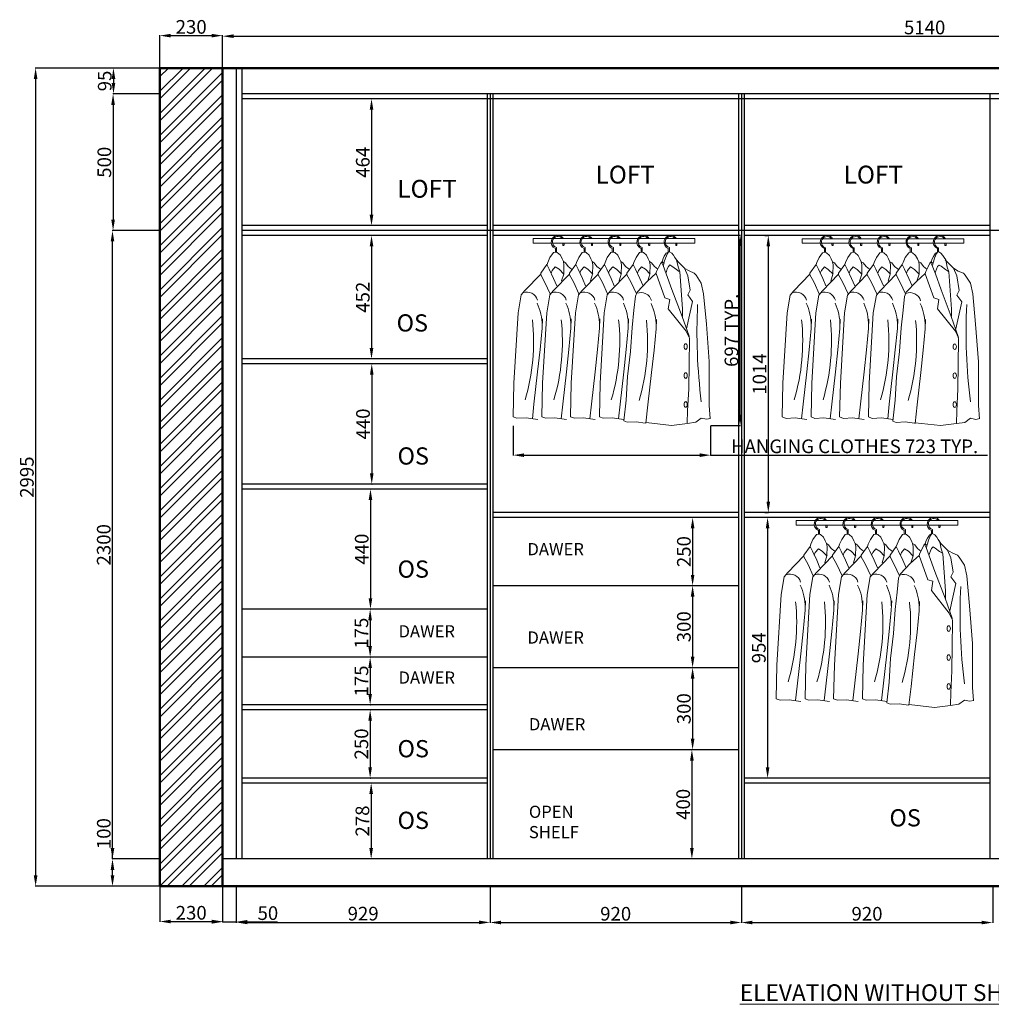
# Model space of a CAD drawing. Units: millimetres. Extents: x -513 to 5600, y -432 to 3172.
# Tile 1 of 2: x -513 to 3044, y -432 to 3172. Entities that reach past the tile are written whole.
import ezdxf

# ---------------------------------------------------------------- set-up
doc = ezdxf.new("R2010")
doc.units = ezdxf.units.MM
for name, color, linetype, lineweight in [('A-ANNO-DIMS', 2, 'Continuous', 18), ('A-ANNO-TEXT', 7, 'Continuous', 18), ('A-FURN', 3, 'Continuous', 25), ('A-FURN-ACCS', 9, 'Continuous', 18), ('A-WALL', 7, 'Continuous', 50), ('A-WALL-PATT', 8, 'Continuous', 13)]:
    doc.layers.add(name, color=color, linetype=linetype, lineweight=lineweight)
doc.styles.get("Standard").update_dxf_attribs({"font": 'arial.ttf'})
doc.dimstyles.new('ISO-25', dxfattribs={"dimtxt": 50, "dimasz": 40, "dimexe": 1.25, "dimexo": 0.625, "dimgap": 0, "dimtad": 1, "dimtxsty": 'Standard', "dimcen": 2.5, "dimclrt": 6, "dimadec": 0, "dimazin": 0, "dimtfac": 1, "dimtmove": 0, "dimatfit": 3, "dimfxl": 1, "dimarcsym": 0})

# ---------------------------------------------------------------- blocks, each defined once
blk = doc.blocks.new('A$C17AF523A')
for p, q in [((221.1, 1060), (113.2, 1060)), ((113.2, 1060), (113.2, 1034.3)), ((216, 1034.3), (113.2, 1034.3)), ((222.5, 1034.3), (378.4, 1034.3)), ((229, 1060), (383.5, 1060)), ((246.1, 1008.9), (246.1, 981.5)), ((285.8, 1060), (336.5, 1060)), ((384.9, 1034.3), (538.6, 1034.3)), ((391.4, 1060), (543.8, 1060)), ((408.5, 1008.9), (408.5, 981.5)), ((545.2, 1034.3), (702.4, 1034.3)), ((551.6, 1060), (707.5, 1060)), ((568.8, 1008.9), (568.8, 981.5)), ((708.9, 1034.3), (856.3, 1034.3)), ((715.4, 1060), (861.4, 1060)), ((732.5, 1008.9), (732.5, 982.4)), ((862.8, 1034.3), (1030.4, 1034.3)), ((869.3, 1060), (1030.4, 1060)), ((886.4, 1008.9), (886.4, 985.5)), ((1030.4, 1060), (1030.4, 1034.3)), ((208.5, 953.2), (196.2, 925.3)), ((228.2, 980.3), (208.5, 953.2)), ((240.6, 982.7), (228.2, 980.3)), ((239.7, 981.5), (239.7, 1004.2)), ((250.4, 980.3), (240.6, 982.7)), ((267.7, 965.5), (250.4, 980.3)), ((277.5, 945), (267.7, 965.5)), ((371.7, 953.2), (359.4, 925.3)), ((391.4, 980.3), (371.7, 953.2)), ((403.7, 982.7), (391.4, 980.3)), ((402.1, 981.5), (402.1, 1004.2)), ((413.6, 980.3), (403.7, 982.7)), ((430.8, 965.5), (413.6, 980.3)), ((440.7, 945), (430.8, 965.5)), ((534.1, 953.2), (521.8, 925.3)), ((553.8, 980.3), (534.1, 953.2)), ((566.1, 982.7), (553.8, 980.3)), ((562.3, 981.5), (562.3, 1004.2)), ((576, 980.3), (566.1, 982.7)), ((593.2, 965.5), (576, 980.3)), ((603.1, 945), (593.2, 965.5)), ((697.3, 953.2), (685, 925.3)), ((717, 980.3), (697.3, 953.2)), ((729.3, 982.7), (717, 980.3)), ((726.1, 981.9), (726.1, 1004.2)), ((739.2, 980.3), (729.3, 982.7)), ((756.4, 965.5), (739.2, 980.3)), ((766.3, 945), (756.4, 965.5)), ((857, 959.7), (850.7, 946.2)), ((868.4, 977.4), (857, 959.7)), ((864.2, 949.2), (857, 928.1)), ((874.7, 975.3), (864.2, 949.2)), ((881.5, 985.8), (868.4, 977.4)), ((881.5, 985.8), (874.7, 975.3)), ((880, 984.9), (880, 1004.2)), ((887.4, 985), (881.5, 985.8)), ((899.2, 978.2), (887.4, 985)), ((910.2, 965.2), (899.2, 978.2)), ((917.7, 953.4), (910.2, 965.2)), ((927, 940.3), (917.7, 953.4)), ((192, 913.2), (156.7, 863.9)), ((204.9, 887.4), (192, 913.2)), ((196.2, 925.3), (192.1, 913)), ((238.9, 899.8), (221.7, 879.3)), ((261.1, 885.9), (238.9, 899.8)), ((284.9, 929.7), (277.5, 945)), ((296.7, 922.6), (284.9, 929.7)), ((284.9, 929.7), (288.4, 912.1)), ((288.4, 912.1), (287.3, 859.2)), ((312, 901.5), (296.7, 922.6)), ((331.5, 886.8), (312, 901.5)), ((355.1, 913.2), (319.8, 863.9)), ((368.1, 887.4), (355.1, 913.2)), ((359.4, 925.3), (355.3, 913)), ((402.1, 899.8), (384.8, 879.3)), ((424.3, 885.9), (402.1, 899.8)), ((448.1, 929.7), (440.7, 945)), ((459.8, 922.6), (448.1, 929.7)), ((448.1, 929.7), (451.6, 912.1)), ((451.6, 912.1), (450.4, 859.2)), ((475.1, 901.5), (459.8, 922.6)), ((494.7, 886.8), (475.1, 901.5)), ((517.5, 913.2), (482.2, 863.9)), ((530.5, 887.4), (517.5, 913.2)), ((521.8, 925.3), (517.7, 913)), ((564.5, 899.8), (547.2, 879.3)), ((586.7, 885.9), (564.5, 899.8)), ((610.5, 929.7), (603.1, 945)), ((622.3, 922.6), (610.5, 929.7)), ((610.5, 929.7), (614, 912.1)), ((614, 912.1), (612.8, 859.2)), ((637.5, 901.5), (622.3, 922.6)), ((657.1, 886.8), (637.5, 901.5)), ((680.7, 913.2), (645.4, 863.9)), ((693.6, 887.4), (680.7, 913.2)), ((685, 925.3), (680.8, 913)), ((727.7, 899.8), (710.4, 879.3)), ((749.8, 885.9), (727.7, 899.8)), ((773.7, 929.7), (766.3, 945)), ((785.4, 922.6), (773.7, 929.7)), ((773.7, 929.7), (777.2, 912.1)), ((777.2, 912.1), (776, 859.2)), ((800.7, 901.5), (785.4, 922.6)), ((820.3, 886.8), (800.7, 901.5)), ((813.7, 874.2), (824.9, 895.9)), ((824.9, 895.9), (837.6, 920.5)), ((837.6, 920.5), (842.9, 928.7)), ((841.4, 926.4), (851.1, 907.8)), ((842.9, 928.7), (854, 920.5)), ((850.7, 946.2), (844.4, 926.4)), ((851.1, 907.8), (868.2, 860.1)), ((852.8, 910), (852.4, 907.5)), ((857, 928.1), (852.8, 910)), ((854, 920.5), (855.5, 919.7)), ((881.1, 902.4), (873.9, 888.1)), ((889.5, 910.4), (881.1, 902.4)), ((900.5, 903.7), (889.5, 910.4)), ((925.8, 885.1), (900.5, 903.7)), ((938.9, 924.4), (924.5, 940.7)), ((927, 940.3), (935.1, 899.5)), ((935.1, 899.5), (944.7, 871.7)), ((971.6, 892.8), (938.9, 924.4)), ((156.7, 859.2), (66.1, 765.1)), ((180.6, 811.5), (154.8, 858.5)), ((156.7, 863.9), (156.7, 859.2)), ((229.6, 834.5), (204.9, 887.4)), ((221.7, 879.3), (215.7, 864.3)), ((319.8, 859.2), (229.2, 765.1)), ((288.2, 858.8), (261.1, 885.9)), ((287.3, 859.2), (275, 820)), ((343.8, 811.5), (317.9, 858.5)), ((319.8, 863.9), (319.8, 859.2)), ((392.8, 834.5), (368.1, 887.4)), ((384.8, 879.3), (378.8, 864.3)), ((482.2, 859.2), (391.6, 765.1)), ((451.4, 858.8), (424.3, 885.9)), ((450.4, 859.2), (438.2, 820)), ((506.2, 811.5), (480.3, 858.5)), ((482.2, 863.9), (482.2, 859.2)), ((555.2, 834.5), (530.5, 887.4)), ((547.2, 879.3), (541.2, 864.3)), ((645.4, 859.2), (554.8, 765.1)), ((613.8, 858.8), (586.7, 885.9)), ((612.8, 859.2), (600.6, 820)), ((669.4, 811.5), (643.5, 858.5)), ((645.4, 863.9), (645.4, 859.2)), ((718.4, 834.5), (693.6, 887.4)), ((710.4, 879.3), (704.4, 864.3)), ((776.9, 858.8), (749.8, 885.9)), ((761.8, 818.2), (810, 862)), ((776, 859.2), (763.8, 820)), ((810, 862), (813.7, 874.2)), ((859.8, 724), (811, 861.6)), ((869.3, 872.5), (867.6, 867)), ((868.2, 860.1), (900.3, 770.6)), ((873.9, 888.1), (869.3, 872.5)), ((942.2, 874.2), (925.8, 885.1)), ((944.7, 871.7), (960, 660.8)), ((970.6, 892.8), (997.5, 876.5)), ((989.8, 849.6), (971.6, 892.8)), ((1004.2, 767.2), (989.8, 849.6)), ((997.5, 876.5), (1027.2, 864)), ((1027.2, 864), (1037.8, 852.5)), ((1037.8, 852.5), (1067.2, 807.9)), ((210.3, 746.9), (180.6, 811.5)), ((247.8, 792.1), (229.6, 834.5)), ((373.4, 746.9), (343.8, 811.5)), ((411, 792.1), (392.8, 834.5)), ((535.8, 746.9), (506.2, 811.5)), ((573.4, 792.1), (555.2, 834.5)), ((699, 746.9), (669.4, 811.5)), ((702.6, 756.9), (761.8, 818.2)), ((736.6, 792.1), (718.4, 834.5)), ((1067.2, 807.9), (1080, 746.6)), ((44.9, 740.4), (27.8, 639.9)), ((66.1, 765.1), (44.9, 740.4)), ((208, 740.4), (190.9, 639.9)), ((229.2, 765.1), (208, 740.4)), ((370.5, 740.4), (353.3, 639.9)), ((391.6, 765.1), (370.5, 740.4)), ((533.6, 740.4), (516.5, 639.9)), ((554.8, 765.1), (533.6, 740.4)), ((685.1, 654), (693.9, 732.8)), ((693.9, 732.8), (702.6, 756.9)), ((900.3, 770.6), (958.5, 619.2)), ((990.7, 740.3), (1004.2, 767.2)), ((1017.6, 702.9), (990.7, 740.3)), ((1080, 746.6), (1096.5, 575.6)), ((888.4, 715.5), (859.8, 724)), ((879.9, 662.5), (888.4, 715.5)), ((984, 548.6), (1017.6, 702.9)), ((27.8, 639.9), (4.2, 240.5)), ((190.9, 639.9), (167.4, 240.5)), ((353.3, 639.9), (329.8, 240.5)), ((516.5, 639.9), (493, 240.5)), ((674.2, 555.5), (685.1, 654)), ((981.6, 535.4), (879.9, 662.5)), ((958.5, 619.2), (997.3, 506.4)), ((960, 660.8), (960, 618.6)), ((163.9, 551.6), (166.2, 604.3)), ((327.1, 551.6), (329.4, 604.3)), ((489.5, 551.6), (491.8, 604.3)), ((652.7, 551.6), (655, 604.3)), ((810.2, 548.7), (812.5, 601.4)), ((1096.5, 575.6), (1112.5, 362.3)), ((152.5, 430.3), (163.9, 551.6)), ((315.7, 430.3), (327.1, 551.6)), ((478.1, 430.3), (489.5, 551.6)), ((641.2, 430.3), (652.7, 551.6)), ((665.4, 419.8), (674.2, 555.5)), ((798.8, 427.4), (810.2, 548.7)), ((998.6, 498.4), (981.6, 535.4)), ((997.3, 506.4), (1000, 487.4)), ((1000, 487.4), (996.4, 208.2)), ((138.7, 304.3), (152.5, 430.3)), ((301.9, 304.3), (315.7, 430.3)), ((464.3, 304.3), (478.1, 430.3)), ((627.5, 304.3), (641.2, 430.3)), ((647.9, 277.5), (665.4, 419.8)), ((785, 301.4), (798.8, 427.4)), ((1112.5, 362.3), (1112.5, 113.9)), ((118.1, 121.1), (138.7, 304.3)), ((281.3, 121.1), (301.9, 304.3)), ((443.7, 121.1), (464.3, 304.3)), ((606.9, 121.1), (627.5, 304.3)), ((764.4, 118.2), (785, 301.4)), ((4.2, 240.5), (0, 49.5)), ((167.4, 240.5), (163.2, 49.5)), ((329.8, 240.5), (325.6, 49.5)), ((493, 240.5), (488.8, 49.5)), ((641.3, 143.9), (647.9, 277.5)), ((996.4, 208.2), (989.7, 82.6)), ((109.2, 38.9), (118.1, 121.1)), ((272.3, 38.9), (281.3, 121.1)), ((434.7, 38.9), (443.7, 121.1)), ((597.9, 38.9), (606.9, 121.1)), ((627.3, 25.8), (641.3, 143.9)), ((752.9, 12.8), (764.4, 118.2)), ((1112.5, 113.9), (1118.2, 39.6)), ((989.7, 82.6), (987.5, 14.7)), ((21.7, 41.4), (0, 49.5)), ((73.3, 43.8), (21.7, 41.4)), ((139.6, 34.7), (73.3, 43.8)), ((184.8, 41.4), (163.2, 49.5)), ((236.5, 43.8), (184.8, 41.4)), ((302.8, 34.7), (236.5, 43.8)), ((347.2, 41.4), (325.6, 49.5)), ((398.9, 43.8), (347.2, 41.4)), ((465.2, 34.7), (398.9, 43.8)), ((510.4, 41.4), (488.8, 49.5)), ((562.1, 43.8), (510.4, 41.4)), ((628.3, 34.7), (562.1, 43.8)), ((646.1, 18.8), (627.3, 25.8)), ((697.8, 21.1), (646.1, 18.8)), ((749.5, 14.1), (697.8, 21.1)), ((754.2, 16.4), (897.4, 0)), ((897.4, 0), (989, 11.7)), ((989, 11.7), (1036, 18.8)), ((1036, 18.8), (1067.2, 42.2)), ((1067.2, 42.2), (1096.9, 35.3)), ((1096.9, 35.3), (1119.7, 39.9))]:
    blk.add_line(p, q)
for centre, radius, start, end in [((253.5, 1040.3), 37.9, 31.4138, 165.4823), ((253.5, 1040.3), 31.5, 38.898, 165.4823), ((415.9, 1040.3), 37.9, 31.4138, 165.4823), ((415.9, 1040.3), 31.5, 38.898, 165.4823), ((576.1, 1040.3), 37.9, 31.4138, 165.4823), ((576.1, 1040.3), 31.5, 38.898, 165.4823), ((739.9, 1040.3), 37.9, 31.4138, 165.4823), ((739.9, 1040.3), 31.5, 38.898, 165.4823), ((893.8, 1040.3), 37.9, 31.4138, 165.4823), ((893.8, 1040.3), 31.5, 38.898, 165.4823), ((254.3, 1040.1), 38.7, 165.4823, 247.8669), ((254.3, 1040.1), 32.3, 165.4823, 255.3823), ((250.7, 1027.2), 31.5, 354.9774, 12.9498), ((285.2, 1024), 3.23, 171.8983, 358.0565), ((250.7, 1027.2), 37.9, 354.9774, 10.7201), ((416.7, 1040.1), 38.7, 165.4823, 247.8669), ((416.7, 1040.1), 32.3, 165.4823, 255.3823), ((413.1, 1027.2), 31.5, 354.9774, 12.9498), ((447.6, 1024), 3.23, 171.8983, 358.0565), ((413.1, 1027.2), 37.9, 354.9774, 10.7201), ((576.9, 1040.1), 38.7, 165.4823, 247.8669), ((576.9, 1040.1), 32.3, 165.4823, 255.3823), ((573.3, 1027.2), 31.5, 354.9774, 12.9498), ((607.9, 1024), 3.23, 171.8983, 358.0565), ((573.3, 1027.2), 37.9, 354.9774, 10.7201), ((740.6, 1040.1), 38.7, 165.4823, 247.8669), ((740.6, 1040.1), 32.3, 165.4823, 255.3823), ((737.1, 1027.2), 31.5, 354.9774, 12.9498), ((771.6, 1024), 3.23, 171.8983, 358.0565), ((737.1, 1027.2), 37.9, 354.9774, 10.7201), ((894.6, 1040.1), 38.7, 165.4823, 247.8669), ((894.6, 1040.1), 32.3, 165.4823, 255.3823), ((891, 1027.2), 31.5, 354.9774, 12.9498), ((925.5, 1024), 3.23, 171.8983, 358.0565), ((891, 1027.2), 37.9, 354.9774, 10.7201), ((78, 694.6), 62.4, 15.7523, 111.1565), ((241.2, 694.6), 62.4, 15.7523, 111.1565), ((403.6, 694.6), 62.4, 15.7523, 111.1565), ((566.7, 694.6), 62.4, 15.7523, 111.1565), ((724.3, 691.7), 62.4, 15.7523, 111.1565), ((-136.4, 567.6), 300.7, 359.9116, 24.988), ((26.8, 567.6), 300.7, 359.9116, 24.988), ((189.2, 567.6), 300.7, 359.9116, 24.988), ((352.4, 567.6), 300.7, 359.9116, 24.988), ((509.9, 564.7), 300.7, 359.9116, 24.988), ((4277.9, 533.2), 3235.4, 177.2767, 187.0811), ((-1056.1, 477.6), 1172.1, 343.5409, 5.9886), ((-892.9, 477.6), 1172.1, 343.5409, 5.9886), ((-567.4, 477.6), 1172.1, 343.5409, 5.9886), ((-409.8, 474.7), 1172.1, 343.5409, 5.9886)]:
    blk.add_arc(centre, radius, start, end)
for centre in [(978.4, 447.7), (978.4, 283.5), (978.4, 119.4)]:
    blk.add_ellipse(centre, major_axis=(0, 16), ratio=0.580645)
blk = doc.blocks.new('*D2')
at = {"layer": 'A-ANNO-DIMS', "color": 0, "lineweight": -2, "transparency": 16777216}
for p, q in [((-0.6, 2995), (-455.7, 2995)), ((-454.4, 2955), (-454.4, 40)), ((-0.6, 0), (-455.7, 0))]:
    blk.add_line(p, q, dxfattribs=at)
at = {"layer": 'A-ANNO-DIMS', "color": 0, "transparency": 16777216}
for points in [[(-461.1, 2955), (-447.8, 2955), (-454.4, 2995)], [(-461.1, 40), (-447.8, 40), (-454.4, 0)]]:
    blk.add_solid(points, dxfattribs=at)
at = {"layer": 'Defpoints', "color": 0, "transparency": 16777216}
for p in [(0, 2995), (0, 0), (-454.4, 0)]:
    blk.add_point(p, dxfattribs=at)
at = {"layer": 'A-ANNO-DIMS', "color": 0, "transparency": 16777216, "insert": (-480, 1497.5), "char_height": 50, "attachment_point": 5, "rotation": 90}
blk.add_mtext('2995', dxfattribs=at)
blk = doc.blocks.new('*D3')
at = {"layer": 'A-ANNO-DIMS', "color": 0, "lineweight": -2, "transparency": 16777216}
for p, q in [((-0.6, 2995), (-170.7, 2995)), ((-169.5, 2955), (-169.5, 2940)), ((-0.6, 2900), (-170.7, 2900))]:
    blk.add_line(p, q, dxfattribs=at)
at = {"layer": 'A-ANNO-DIMS', "color": 0, "transparency": 16777216}
for points in [[(-176.1, 2955), (-162.8, 2955), (-169.5, 2995)], [(-176.1, 2940), (-162.8, 2940), (-169.5, 2900)]]:
    blk.add_solid(points, dxfattribs=at)
at = {"layer": 'Defpoints', "color": 0, "transparency": 16777216}
for p in [(0, 2995), (-169.5, 2900), (0, 2900)]:
    blk.add_point(p, dxfattribs=at)
at = {"layer": 'A-ANNO-DIMS', "color": 0, "transparency": 16777216, "insert": (-195, 2947.5), "char_height": 50, "attachment_point": 5, "rotation": 90}
blk.add_mtext('95', dxfattribs=at)
blk = doc.blocks.new('*D4')
at = {"layer": 'A-ANNO-DIMS', "color": 0, "lineweight": -2, "transparency": 16777216}
for p, q in [((-0.6, 2900), (-172.2, 2900)), ((-170.9, 2860), (-170.9, 2440)), ((-0.6, 2400), (-172.2, 2400))]:
    blk.add_line(p, q, dxfattribs=at)
at = {"layer": 'A-ANNO-DIMS', "color": 0, "transparency": 16777216}
for points in [[(-177.6, 2860), (-164.3, 2860), (-170.9, 2900)], [(-177.6, 2440), (-164.3, 2440), (-170.9, 2400)]]:
    blk.add_solid(points, dxfattribs=at)
at = {"layer": 'Defpoints', "color": 0, "transparency": 16777216}
for p in [(0, 2900), (-170.9, 2400), (0, 2400)]:
    blk.add_point(p, dxfattribs=at)
at = {"layer": 'A-ANNO-DIMS', "color": 0, "transparency": 16777216, "insert": (-196.5, 2650), "char_height": 50, "attachment_point": 5, "rotation": 90}
blk.add_mtext('500', dxfattribs=at)
blk = doc.blocks.new('*D5')
at = {"layer": 'A-ANNO-DIMS', "color": 0, "lineweight": -2, "transparency": 16777216}
for p, q in [((-0.6, 2400), (-174.3, 2400)), ((-173, 140), (-173, 2360)), ((-0.6, 100), (-174.3, 100))]:
    blk.add_line(p, q, dxfattribs=at)
at = {"layer": 'A-ANNO-DIMS', "color": 0, "transparency": 16777216}
for points in [[(-179.7, 2360), (-166.4, 2360), (-173, 2400)], [(-179.7, 140), (-166.4, 140), (-173, 100)]]:
    blk.add_solid(points, dxfattribs=at)
at = {"layer": 'Defpoints', "color": 0, "transparency": 16777216}
for p in [(-173, 2400), (0, 2400), (0, 100)]:
    blk.add_point(p, dxfattribs=at)
at = {"layer": 'A-ANNO-DIMS', "color": 0, "transparency": 16777216, "insert": (-198.6, 1250), "char_height": 50, "attachment_point": 5, "rotation": 90}
blk.add_mtext('2300', dxfattribs=at)
blk = doc.blocks.new('*D6')
at = {"layer": 'A-ANNO-DIMS', "color": 0, "lineweight": -2, "transparency": 16777216}
for p, q in [((-173, 100), (-173, 245.6)), ((-0.6, 100), (-174.2, 100)), ((-173, 40), (-173, 60)), ((-0.6, 0), (-174.2, 0))]:
    blk.add_line(p, q, dxfattribs=at)
at = {"layer": 'A-ANNO-DIMS', "color": 0, "transparency": 16777216}
for points in [[(-179.7, 60), (-166.3, 60), (-173, 100)], [(-179.7, 40), (-166.3, 40), (-173, 0)]]:
    blk.add_solid(points, dxfattribs=at)
at = {"layer": 'Defpoints', "color": 0, "transparency": 16777216}
for p in [(-173, 100), (0, 100), (0, 0)]:
    blk.add_point(p, dxfattribs=at)
at = {"layer": 'A-ANNO-DIMS', "color": 0, "transparency": 16777216, "insert": (-198.5, 192.8), "char_height": 50, "attachment_point": 5, "rotation": 90}
blk.add_mtext('100', dxfattribs=at)
blk = doc.blocks.new('*D7')
at = {"layer": 'A-ANNO-DIMS', "color": 0, "lineweight": -2, "transparency": 16777216}
for p, q in [((0, -0.6), (0, -130.2)), ((230, -0.6), (230, -130.2)), ((40, -128.9), (190, -128.9))]:
    blk.add_line(p, q, dxfattribs=at)
at = {"layer": 'A-ANNO-DIMS', "color": 0, "transparency": 16777216}
for points in [[(40, -122.3), (40, -135.6), (0, -128.9)], [(190, -122.3), (190, -135.6), (230, -128.9)]]:
    blk.add_solid(points, dxfattribs=at)
at = {"layer": 'Defpoints', "color": 0, "transparency": 16777216}
for p in [(0, 0), (230, 0), (230, -128.9)]:
    blk.add_point(p, dxfattribs=at)
at = {"layer": 'A-ANNO-DIMS', "color": 0, "transparency": 16777216, "insert": (115, -103.4), "char_height": 50, "attachment_point": 5}
blk.add_mtext('230', dxfattribs=at)
blk = doc.blocks.new('*D8')
at = {"layer": 'A-ANNO-DIMS', "color": 0, "lineweight": -2, "transparency": 16777216}
for p, q in [((230, -0.6), (230, -131.4)), ((280, -0.6), (280, -131.4)), ((190, -130.1), (150, -130.1)), ((230, -130.1), (280, -130.1)), ((320, -130.1), (431.5, -130.1))]:
    blk.add_line(p, q, dxfattribs=at)
at = {"layer": 'A-ANNO-DIMS', "color": 0, "transparency": 16777216}
for points in [[(190, -123.4), (190, -136.8), (230, -130.1)], [(320, -123.4), (320, -136.8), (280, -130.1)]]:
    blk.add_solid(points, dxfattribs=at)
at = {"layer": 'Defpoints', "color": 0, "transparency": 16777216}
for p in [(230, 0), (280, 0), (280, -130.1)]:
    blk.add_point(p, dxfattribs=at)
at = {"layer": 'A-ANNO-DIMS', "color": 0, "transparency": 16777216, "insert": (395.7, -104.6), "char_height": 50, "attachment_point": 5}
blk.add_mtext('50', dxfattribs=at)
blk = doc.blocks.new('*D9')
at = {"layer": 'A-ANNO-DIMS', "color": 0, "lineweight": -2, "transparency": 16777216}
for p, q in [((280, -0.6), (280, -133.3)), ((1209, -0.6), (1209, -133.3)), ((320, -132), (1169, -132))]:
    blk.add_line(p, q, dxfattribs=at)
at = {"layer": 'A-ANNO-DIMS', "color": 0, "transparency": 16777216}
for points in [[(320, -125.4), (320, -138.7), (280, -132)], [(1169, -125.4), (1169, -138.7), (1209, -132)]]:
    blk.add_solid(points, dxfattribs=at)
at = {"layer": 'Defpoints', "color": 0, "transparency": 16777216}
for p in [(280, 0), (1209, 0), (1209, -132)]:
    blk.add_point(p, dxfattribs=at)
at = {"layer": 'A-ANNO-DIMS', "color": 0, "transparency": 16777216, "insert": (744.5, -106.5), "char_height": 50, "attachment_point": 5}
blk.add_mtext('929', dxfattribs=at)
blk = doc.blocks.new('*D10')
at = {"layer": 'A-ANNO-DIMS', "color": 0, "lineweight": -2, "transparency": 16777216}
for p, q in [((1209, -0.6), (1209, -133.8)), ((2129, -0.6), (2129, -133.8)), ((1249, -132.5), (2089, -132.5))]:
    blk.add_line(p, q, dxfattribs=at)
at = {"layer": 'A-ANNO-DIMS', "color": 0, "transparency": 16777216}
for points in [[(1249, -125.9), (1249, -139.2), (1209, -132.5)], [(2089, -125.9), (2089, -139.2), (2129, -132.5)]]:
    blk.add_solid(points, dxfattribs=at)
at = {"layer": 'Defpoints', "color": 0, "transparency": 16777216}
for p in [(1209, 0), (2129, 0), (2129, -132.5)]:
    blk.add_point(p, dxfattribs=at)
at = {"layer": 'A-ANNO-DIMS', "color": 0, "transparency": 16777216, "insert": (1669, -107), "char_height": 50, "attachment_point": 5}
blk.add_mtext('920', dxfattribs=at)
blk = doc.blocks.new('*D11')
at = {"layer": 'A-ANNO-DIMS', "color": 0, "lineweight": -2, "transparency": 16777216}
for p, q in [((2129, -0.6), (2129, -133.8)), ((3049, -0.6), (3049, -133.8)), ((2169, -132.6), (3009, -132.6))]:
    blk.add_line(p, q, dxfattribs=at)
at = {"layer": 'A-ANNO-DIMS', "color": 0, "transparency": 16777216}
for points in [[(2169, -125.9), (2169, -139.2), (2129, -132.6)], [(3009, -125.9), (3009, -139.2), (3049, -132.6)]]:
    blk.add_solid(points, dxfattribs=at)
at = {"layer": 'Defpoints', "color": 0, "transparency": 16777216}
for p in [(2129, 0), (3049, 0), (3049, -132.6)]:
    blk.add_point(p, dxfattribs=at)
at = {"layer": 'A-ANNO-DIMS', "color": 0, "transparency": 16777216, "insert": (2589, -107), "char_height": 50, "attachment_point": 5}
blk.add_mtext('920', dxfattribs=at)
blk = doc.blocks.new('*D16')
at = {"layer": 'A-ANNO-DIMS', "color": 0, "lineweight": -2, "transparency": 16777216}
for p, q in [((775.8, 2882), (776.4, 2882)), ((775.1, 2842), (775.1, 2458)), ((775.8, 2418), (776.4, 2418))]:
    blk.add_line(p, q, dxfattribs=at)
at = {"layer": 'A-ANNO-DIMS', "color": 0, "transparency": 16777216}
for points in [[(768.5, 2842), (781.8, 2842), (775.1, 2882)], [(768.5, 2458), (781.8, 2458), (775.1, 2418)]]:
    blk.add_solid(points, dxfattribs=at)
at = {"layer": 'Defpoints', "color": 0, "transparency": 16777216}
for p in [(775.1, 2882), (775.1, 2418), (775.1, 2418)]:
    blk.add_point(p, dxfattribs=at)
at = {"layer": 'A-ANNO-DIMS', "color": 0, "transparency": 16777216, "insert": (749.6, 2650), "char_height": 50, "attachment_point": 5, "rotation": 90}
blk.add_mtext('464', dxfattribs=at)
blk = doc.blocks.new('*D17')
at = {"layer": 'A-ANNO-DIMS', "color": 0, "lineweight": -2, "transparency": 16777216}
for p, q in [((775.8, 2382), (776.4, 2382)), ((775.1, 2342), (775.1, 1970)), ((775.8, 1930), (776.4, 1930))]:
    blk.add_line(p, q, dxfattribs=at)
at = {"layer": 'A-ANNO-DIMS', "color": 0, "transparency": 16777216}
for points in [[(768.5, 2342), (781.8, 2342), (775.1, 2382)], [(768.5, 1970), (781.8, 1970), (775.1, 1930)]]:
    blk.add_solid(points, dxfattribs=at)
at = {"layer": 'Defpoints', "color": 0, "transparency": 16777216}
for p in [(775.1, 2382), (775.1, 1930), (775.1, 1930)]:
    blk.add_point(p, dxfattribs=at)
at = {"layer": 'A-ANNO-DIMS', "color": 0, "transparency": 16777216, "insert": (749.6, 2156), "char_height": 50, "attachment_point": 5, "rotation": 90}
blk.add_mtext('452', dxfattribs=at)
blk = doc.blocks.new('*D18')
at = {"layer": 'A-ANNO-DIMS', "color": 0, "lineweight": -2, "transparency": 16777216}
for p, q in [((775.8, 1912), (777.3, 1912)), ((776, 1872), (776, 1512)), ((775.8, 1472), (777.3, 1472))]:
    blk.add_line(p, q, dxfattribs=at)
at = {"layer": 'A-ANNO-DIMS', "color": 0, "transparency": 16777216}
for points in [[(769.4, 1872), (782.7, 1872), (776, 1912)], [(769.4, 1512), (782.7, 1512), (776, 1472)]]:
    blk.add_solid(points, dxfattribs=at)
at = {"layer": 'Defpoints', "color": 0, "transparency": 16777216}
for p in [(775.1, 1912), (775.1, 1472), (776, 1472)]:
    blk.add_point(p, dxfattribs=at)
at = {"layer": 'A-ANNO-DIMS', "color": 0, "transparency": 16777216, "insert": (750.5, 1692), "char_height": 50, "attachment_point": 5, "rotation": 90}
blk.add_mtext('440', dxfattribs=at)
blk = doc.blocks.new('*D19')
at = {"layer": 'A-ANNO-DIMS', "color": 0, "lineweight": -2, "transparency": 16777216}
for p, q in [((775.4, 1454), (770.1, 1454)), ((771.3, 1414), (771.3, 1054)), ((775.4, 1014), (770.1, 1014))]:
    blk.add_line(p, q, dxfattribs=at)
at = {"layer": 'A-ANNO-DIMS', "color": 0, "transparency": 16777216}
for points in [[(764.7, 1414), (778, 1414), (771.3, 1454)], [(764.7, 1054), (778, 1054), (771.3, 1014)]]:
    blk.add_solid(points, dxfattribs=at)
at = {"layer": 'Defpoints', "color": 0, "transparency": 16777216}
for p in [(776, 1454), (771.3, 1014), (776, 1014)]:
    blk.add_point(p, dxfattribs=at)
at = {"layer": 'A-ANNO-DIMS', "color": 0, "transparency": 16777216, "insert": (745.8, 1234), "char_height": 50, "attachment_point": 5, "rotation": 90}
blk.add_mtext('440', dxfattribs=at)
blk = doc.blocks.new('*D20')
at = {"layer": 'A-ANNO-DIMS', "color": 0, "lineweight": -2, "transparency": 16777216}
for p, q in [((770.7, 1014), (771.3, 1014)), ((770.1, 974), (770.1, 879)), ((770.7, 839), (771.3, 839))]:
    blk.add_line(p, q, dxfattribs=at)
at = {"layer": 'A-ANNO-DIMS', "color": 0, "transparency": 16777216}
for points in [[(763.4, 974), (776.7, 974), (770.1, 1014)], [(763.4, 879), (776.7, 879), (770.1, 839)]]:
    blk.add_solid(points, dxfattribs=at)
at = {"layer": 'Defpoints', "color": 0, "transparency": 16777216}
for p in [(770.1, 1014), (770.1, 839), (770.1, 839)]:
    blk.add_point(p, dxfattribs=at)
at = {"layer": 'A-ANNO-DIMS', "color": 0, "transparency": 16777216, "insert": (744.6, 926.5), "char_height": 50, "attachment_point": 5, "rotation": 90}
blk.add_mtext('175', dxfattribs=at)
blk = doc.blocks.new('*D21')
at = {"layer": 'A-ANNO-DIMS', "color": 0, "lineweight": -2, "transparency": 16777216}
for p, q in [((770.7, 839), (771.3, 839)), ((770.1, 799), (770.1, 704)), ((770.7, 664), (771.3, 664))]:
    blk.add_line(p, q, dxfattribs=at)
at = {"layer": 'A-ANNO-DIMS', "color": 0, "transparency": 16777216}
for points in [[(763.4, 799), (776.7, 799), (770.1, 839)], [(763.4, 704), (776.7, 704), (770.1, 664)]]:
    blk.add_solid(points, dxfattribs=at)
at = {"layer": 'Defpoints', "color": 0, "transparency": 16777216}
for p in [(770.1, 839), (770.1, 664), (770.1, 664)]:
    blk.add_point(p, dxfattribs=at)
at = {"layer": 'A-ANNO-DIMS', "color": 0, "transparency": 16777216, "insert": (744.6, 751.5), "char_height": 50, "attachment_point": 5, "rotation": 90}
blk.add_mtext('175', dxfattribs=at)
blk = doc.blocks.new('*D22')
at = {"layer": 'A-ANNO-DIMS', "color": 0, "lineweight": -2, "transparency": 16777216}
for p, q in [((770.7, 646), (771.3, 646)), ((770.1, 606), (770.1, 436)), ((770.7, 396), (771.3, 396))]:
    blk.add_line(p, q, dxfattribs=at)
at = {"layer": 'A-ANNO-DIMS', "color": 0, "transparency": 16777216}
for points in [[(763.4, 606), (776.7, 606), (770.1, 646)], [(763.4, 436), (776.7, 436), (770.1, 396)]]:
    blk.add_solid(points, dxfattribs=at)
at = {"layer": 'Defpoints', "color": 0, "transparency": 16777216}
for p in [(770.1, 646), (770.1, 396), (770.1, 396)]:
    blk.add_point(p, dxfattribs=at)
at = {"layer": 'A-ANNO-DIMS', "color": 0, "transparency": 16777216, "insert": (744.6, 521), "char_height": 50, "attachment_point": 5, "rotation": 90}
blk.add_mtext('250', dxfattribs=at)
blk = doc.blocks.new('*D23')
at = {"layer": 'A-ANNO-DIMS', "color": 0, "lineweight": -2, "transparency": 16777216}
for p, q in [((774.5, 378), (775.1, 378)), ((773.8, 338), (773.8, 140)), ((774.5, 100), (775.1, 100))]:
    blk.add_line(p, q, dxfattribs=at)
at = {"layer": 'A-ANNO-DIMS', "color": 0, "transparency": 16777216}
for points in [[(767.2, 338), (780.5, 338), (773.8, 378)], [(767.2, 140), (780.5, 140), (773.8, 100)]]:
    blk.add_solid(points, dxfattribs=at)
at = {"layer": 'Defpoints', "color": 0, "transparency": 16777216}
for p in [(773.8, 378), (773.8, 100), (773.8, 100)]:
    blk.add_point(p, dxfattribs=at)
at = {"layer": 'A-ANNO-DIMS', "color": 0, "transparency": 16777216, "insert": (748.3, 239), "char_height": 50, "attachment_point": 5, "rotation": 90}
blk.add_mtext('278', dxfattribs=at)
blk = doc.blocks.new('*D24')
at = {"layer": 'A-ANNO-DIMS', "color": 0, "lineweight": -2, "transparency": 16777216}
for p, q in [((1951.2, 1350), (1951.8, 1350)), ((1950.6, 1310), (1950.6, 1140)), ((1951.2, 1100), (1951.8, 1100))]:
    blk.add_line(p, q, dxfattribs=at)
at = {"layer": 'A-ANNO-DIMS', "color": 0, "transparency": 16777216}
for points in [[(1943.9, 1310), (1957.2, 1310), (1950.6, 1350)], [(1943.9, 1140), (1957.2, 1140), (1950.6, 1100)]]:
    blk.add_solid(points, dxfattribs=at)
at = {"layer": 'Defpoints', "color": 0, "transparency": 16777216}
for p in [(1950.6, 1350), (1950.6, 1100), (1950.6, 1100)]:
    blk.add_point(p, dxfattribs=at)
at = {"layer": 'A-ANNO-DIMS', "color": 0, "transparency": 16777216, "insert": (1925, 1225), "char_height": 50, "attachment_point": 5, "rotation": 90}
blk.add_mtext('250', dxfattribs=at)
blk = doc.blocks.new('*D25')
at = {"layer": 'A-ANNO-DIMS', "color": 0, "lineweight": -2, "transparency": 16777216}
for p, q in [((1951.2, 1100), (1951.8, 1100)), ((1950.6, 1060), (1950.6, 840)), ((1951.2, 800), (1951.8, 800))]:
    blk.add_line(p, q, dxfattribs=at)
at = {"layer": 'A-ANNO-DIMS', "color": 0, "transparency": 16777216}
for points in [[(1943.9, 1060), (1957.2, 1060), (1950.6, 1100)], [(1943.9, 840), (1957.2, 840), (1950.6, 800)]]:
    blk.add_solid(points, dxfattribs=at)
at = {"layer": 'Defpoints', "color": 0, "transparency": 16777216}
for p in [(1950.6, 1100), (1950.6, 800), (1950.6, 800)]:
    blk.add_point(p, dxfattribs=at)
at = {"layer": 'A-ANNO-DIMS', "color": 0, "transparency": 16777216, "insert": (1925, 950), "char_height": 50, "attachment_point": 5, "rotation": 90}
blk.add_mtext('300', dxfattribs=at)
blk = doc.blocks.new('*D26')
at = {"layer": 'A-ANNO-DIMS', "color": 0, "lineweight": -2, "transparency": 16777216}
for p, q in [((1951.2, 800), (1951.8, 800)), ((1950.6, 760), (1950.6, 540)), ((1951.2, 500), (1951.8, 500))]:
    blk.add_line(p, q, dxfattribs=at)
at = {"layer": 'A-ANNO-DIMS', "color": 0, "transparency": 16777216}
for points in [[(1943.9, 760), (1957.2, 760), (1950.6, 800)], [(1943.9, 540), (1957.2, 540), (1950.6, 500)]]:
    blk.add_solid(points, dxfattribs=at)
at = {"layer": 'Defpoints', "color": 0, "transparency": 16777216}
for p in [(1950.6, 800), (1950.6, 500), (1950.6, 500)]:
    blk.add_point(p, dxfattribs=at)
at = {"layer": 'A-ANNO-DIMS', "color": 0, "transparency": 16777216, "insert": (1925, 650), "char_height": 50, "attachment_point": 5, "rotation": 90}
blk.add_mtext('300', dxfattribs=at)
blk = doc.blocks.new('*D27')
at = {"layer": 'A-ANNO-DIMS', "color": 0, "lineweight": -2, "transparency": 16777216}
for p, q in [((1949.9, 500), (1946.7, 500)), ((1948, 460), (1948, 140)), ((1949.9, 100), (1946.7, 100))]:
    blk.add_line(p, q, dxfattribs=at)
at = {"layer": 'A-ANNO-DIMS', "color": 0, "transparency": 16777216}
for points in [[(1941.3, 460), (1954.6, 460), (1948, 500)], [(1941.3, 140), (1954.6, 140), (1948, 100)]]:
    blk.add_solid(points, dxfattribs=at)
at = {"layer": 'Defpoints', "color": 0, "transparency": 16777216}
for p in [(1950.6, 500), (1948, 100), (1950.6, 100)]:
    blk.add_point(p, dxfattribs=at)
at = {"layer": 'A-ANNO-DIMS', "color": 0, "transparency": 16777216, "insert": (1922.4, 300), "char_height": 50, "attachment_point": 5, "rotation": 90}
blk.add_mtext('400', dxfattribs=at)
blk = doc.blocks.new('*D28')
at = {"layer": 'A-ANNO-DIMS', "color": 0, "lineweight": -2, "transparency": 16777216}
for p, q in [((2225.6, 1350), (2226.3, 1350)), ((2225, 1310), (2225, 436)), ((2225.6, 396), (2226.3, 396))]:
    blk.add_line(p, q, dxfattribs=at)
at = {"layer": 'A-ANNO-DIMS', "color": 0, "transparency": 16777216}
for points in [[(2218.4, 1310), (2231.7, 1310), (2225, 1350)], [(2218.4, 436), (2231.7, 436), (2225, 396)]]:
    blk.add_solid(points, dxfattribs=at)
at = {"layer": 'Defpoints', "color": 0, "transparency": 16777216}
for p in [(2225, 1350), (2225, 396), (2225, 396)]:
    blk.add_point(p, dxfattribs=at)
at = {"layer": 'A-ANNO-DIMS', "color": 0, "transparency": 16777216, "insert": (2199.5, 873), "char_height": 50, "attachment_point": 5, "rotation": 90}
blk.add_mtext('954', dxfattribs=at)
blk = doc.blocks.new('*D29')
at = {"layer": 'A-ANNO-DIMS', "color": 0, "lineweight": -2, "transparency": 16777216}
for p, q in [((2214.6, 2382), (2228.9, 2382)), ((2227.6, 2342), (2227.6, 1408)), ((2214.6, 1368), (2228.9, 1368))]:
    blk.add_line(p, q, dxfattribs=at)
at = {"layer": 'A-ANNO-DIMS', "color": 0, "transparency": 16777216}
for points in [[(2221, 2342), (2234.3, 2342), (2227.6, 2382)], [(2221, 1408), (2234.3, 1408), (2227.6, 1368)]]:
    blk.add_solid(points, dxfattribs=at)
at = {"layer": 'Defpoints', "color": 0, "transparency": 16777216}
for p in [(2213.9, 2382), (2213.9, 1368), (2227.6, 1368)]:
    blk.add_point(p, dxfattribs=at)
at = {"layer": 'A-ANNO-DIMS', "color": 0, "transparency": 16777216, "insert": (2202.1, 1875), "char_height": 50, "attachment_point": 5, "rotation": 90}
blk.add_mtext('1014', dxfattribs=at)
blk = doc.blocks.new('*D39')
at = {"layer": 'A-ANNO-DIMS', "color": 0, "lineweight": -2, "transparency": 16777216}
for p, q in [((0, 2995.6), (0, 3114.7)), ((40, 3113.4), (190, 3113.4)), ((230, 2995.6), (230, 3114.7))]:
    blk.add_line(p, q, dxfattribs=at)
at = {"layer": 'A-ANNO-DIMS', "color": 0, "transparency": 16777216}
for points in [[(40, 3120.1), (40, 3106.8), (0, 3113.4)], [(190, 3120.1), (190, 3106.8), (230, 3113.4)]]:
    blk.add_solid(points, dxfattribs=at)
at = {"layer": 'Defpoints', "color": 0, "transparency": 16777216}
for p in [(230, 3113.4), (0, 2995), (230, 2995)]:
    blk.add_point(p, dxfattribs=at)
at = {"layer": 'A-ANNO-DIMS', "color": 0, "transparency": 16777216, "insert": (115, 3139), "char_height": 50, "attachment_point": 5}
blk.add_mtext('230', dxfattribs=at)
blk = doc.blocks.new('*D40')
at = {"layer": 'A-ANNO-DIMS', "color": 0, "lineweight": -2, "transparency": 16777216}
for p, q in [((230, 2995.6), (230, 3112.7)), ((270, 3111.4), (5330, 3111.4)), ((5370, 2995.6), (5370, 3112.7))]:
    blk.add_line(p, q, dxfattribs=at)
at = {"layer": 'A-ANNO-DIMS', "color": 0, "transparency": 16777216}
for points in [[(270, 3118.1), (270, 3104.8), (230, 3111.4)], [(5330, 3118.1), (5330, 3104.8), (5370, 3111.4)]]:
    blk.add_solid(points, dxfattribs=at)
at = {"layer": 'Defpoints', "color": 0, "transparency": 16777216}
for p in [(5370, 3111.4), (230, 2995), (5370, 2995)]:
    blk.add_point(p, dxfattribs=at)
at = {"layer": 'A-ANNO-DIMS', "color": 0, "transparency": 16777216, "insert": (2800, 3136.9), "char_height": 50, "attachment_point": 5}
blk.add_mtext('5140', dxfattribs=at)
blk = doc.blocks.new('*D42')
at = {"layer": 'A-ANNO-DIMS', "color": 0, "lineweight": -2, "transparency": 16777216}
for p, q in [((1293.6, 1685.8), (1293.6, 1576.7)), ((2016.4, 1685.8), (2016.4, 1576.7)), ((1333.6, 1578), (1976.4, 1578)), ((2016.4, 1578), (3030.6, 1578))]:
    blk.add_line(p, q, dxfattribs=at)
at = {"layer": 'A-ANNO-DIMS', "color": 0, "transparency": 16777216}
for points in [[(1333.6, 1584.6), (1333.6, 1571.3), (1293.6, 1578)], [(1976.4, 1584.6), (1976.4, 1571.3), (2016.4, 1578)]]:
    blk.add_solid(points, dxfattribs=at)
at = {"layer": 'Defpoints', "color": 0, "transparency": 16777216}
for p in [(1293.6, 1686.4), (2016.4, 1686.4), (2016.4, 1578)]:
    blk.add_point(p, dxfattribs=at)
at = {"layer": 'A-ANNO-DIMS', "color": 6, "transparency": 16777216, "insert": (2543.5, 1603.9), "char_height": 50, "attachment_point": 5}
blk.add_mtext('HANGING CLOTHES 723 TYP.', dxfattribs=at)
blk = doc.blocks.new('*D43')
at = {"layer": 'A-ANNO-DIMS', "color": 0, "lineweight": -2, "transparency": 16777216}
for p, q in [((2017, 2383.6), (2126, 2383.6)), ((2124.8, 1726.4), (2124.8, 2343.6)), ((2017, 1686.4), (2126, 1686.4))]:
    blk.add_line(p, q, dxfattribs=at)
at = {"layer": 'A-ANNO-DIMS', "color": 0, "transparency": 16777216}
for points in [[(2118.1, 2343.6), (2131.4, 2343.6), (2124.8, 2383.6)], [(2118.1, 1726.4), (2131.4, 1726.4), (2124.8, 1686.4)]]:
    blk.add_solid(points, dxfattribs=at)
at = {"layer": 'Defpoints', "color": 0, "transparency": 16777216}
for p in [(2016.4, 2383.6), (2124.8, 2383.6), (2016.4, 1686.4)]:
    blk.add_point(p, dxfattribs=at)
at = {"layer": 'A-ANNO-DIMS', "color": 6, "transparency": 16777216, "insert": (2099.2, 2035), "char_height": 50, "attachment_point": 5, "rotation": 90}
blk.add_mtext('697 TYP.', dxfattribs=at)

msp = doc.modelspace()

# ---------------------------------------------------------------- hatches: boundary and pattern name
at = {"layer": 'A-WALL-PATT'}
h = msp.add_hatch(dxfattribs=at)
h.set_pattern_fill('ANSI32', color=256, scale=6)
h.paths.add_polyline_path([(230, 2995), (0, 2995), (0, 0), (230, 0)])

# ---------------------------------------------------------------- linework, layer by layer
at = {"layer": 'A-FURN'}
for p, q in [((280, 2995), (280, 100)), ((300, 2995), (300, 100)), ((5370, 2900), (300, 2900)), ((1199, 2900), (1199, 100)), ((1209, 2900), (1209, 100)), ((1219, 2900), (1219, 100)), ((2119, 2900), (2119, 100)), ((2129, 2900), (2129, 100)), ((2139, 2900), (2139, 100)), ((3039, 2900), (3039, 100)), ((5370, 2882), (300, 2882)), ((1199, 2418), (300, 2418)), ((2119, 2418), (1219, 2418)), ((3039, 2418), (2139, 2418)), ((5309, 2400), (300, 2400)), ((1199, 2382), (300, 2382)), ((2119, 2382), (1219, 2382)), ((3039, 2382), (2139, 2382)), ((1199, 1930), (300, 1930)), ((1199, 1912), (300, 1912)), ((1199, 1472), (300, 1472)), ((1199, 1454), (300, 1454)), ((2119, 1368), (1219, 1368)), ((2119, 1350), (1219, 1350)), ((3039, 1368), (2139, 1368)), ((3039, 1350), (2139, 1350)), ((2119, 1100), (1219, 1100)), ((1199, 1014), (300, 1014)), ((1199, 839), (300, 839)), ((2119, 800), (1219, 800)), ((1199, 664), (300, 664)), ((1199, 646), (300, 646)), ((2119, 500), (1219, 500)), ((1199, 396), (300, 396)), ((1199, 378), (300, 378)), ((3039, 396), (2139, 396)), ((3039, 378), (2139, 378)), ((5370, 100), (230, 100))]:
    msp.add_line(p, q, dxfattribs=at)
at = {"layer": 'A-WALL'}
for p, q in [((5600, 2995), (0, 2995)), ((0, 2995), (0, 0)), ((230, 2995), (230, 0)), ((0, 0), (5600, 0))]:
    msp.add_line(p, q, dxfattribs=at)

# ---------------------------------------------------------------- block references
at = {"layer": 'A-FURN-ACCS', "xscale": 0.6455188424335829, "yscale": 0.6455188424335829, "zscale": 0.6455188424335829}
for p in [(1293.583, 1686.397), (2278.676, 1686.005), (2256.662, 654.397)]:
    msp.add_blockref('A$C17AF523A', p, dxfattribs=at)

# ---------------------------------------------------------------- texts
at = {"layer": 'A-ANNO-TEXT', "char_height": 65.3441, "width": 459.1587, "attachment_point": 1}
for insert in [(1595.295, 2637.513), (2503.545, 2637.513), (869.739, 2585.571)]:
    msp.add_mtext('{LOFT}', dxfattribs=dict(at, insert=insert))
at = {"layer": 'A-ANNO-TEXT', "attachment_point": 1}
for s, width, gutter_width, insert, char_height in [('{OS}', 5219.99715, 314.97, (866.973, 2093.454), 62.994), ('{OS}', 5219.99715, 314.97, (870.426, 1606.522), 62.994), ('{DAWER}', 7433.56022, 222.871, (1345.924, 1256.329), 44.5743), ('{OS}', 5219.99715, 314.97, (870.426, 1192.538), 62.994), ('{DAWER}', 7433.56022, 222.871, (874.087, 955.585), 44.5743), ('{DAWER}', 7433.56022, 222.871, (1345.924, 932.877), 44.5743), ('{DAWER}', 7433.56022, 222.871, (874.087, 786.262), 44.5743), ('{DAWER}', 7433.56022, 222.871, (1351.244, 615.451), 44.5743), ('{OS}', 5219.99715, 314.97, (870.426, 535.187), 62.994), ('{OPEN\\PSHELF}', 7433.56022, 222.871, (1351.244, 295.018), 44.5743), ('{OS}', 5219.99715, 314.97, (870.426, 272.997), 62.994), ('{OS}', 5219.99715, 314.97, (2671.154, 282.173), 62.994), ('{\\LELEVATION WITHOUT SHUTTER}', 10157.59804, 304.543, (2123.311, -358.773), 60.90856)]:
    msp.add_mtext_dynamic_manual_height_columns(s, width=width, gutter_width=gutter_width, heights=[0], dxfattribs=dict(at, insert=insert, char_height=char_height))

# ---------------------------------------------------------------- dimensions: what is measured, and where the dimension line sits
at = {"layer": 'A-ANNO-DIMS'}
for base, p1, p2, picture, middle in [((230, 3113.449), (0, 2995), (230, 2995), '*D39', (115, 3138.995)), ((5370, 3111.419), (230, 2995), (5370, 2995), '*D40', (2800, 3136.948)), ((230, -128.924), (0, 0), (230, 0), '*D7', (115, -103.379)), ((280, -130.109), (230, 0), (280, 0), '*D8', (395.726, -104.581)), ((1209, -132.033), (280, 0), (1209, 0), '*D9', (744.5, -106.504)), ((2129, -132.523), (1209, 0), (2129, 0), '*D10', (1669, -106.994)), ((3049, -132.558), (2129, 0), (3049, 0), '*D11', (2589, -107.029))]:
    dim = msp.add_linear_dim(base=base, p1=p1, p2=p2, dimstyle='ISO-25', override={"dimclrd": 0, "dimclre": 0, "dimclrt": 0}, dxfattribs=at)
    dim.commit()
    dim.dimension.update_dxf_attribs({"geometry": picture, "text_midpoint": middle})
for base, p1, p2, picture, middle in [((-454.446, 0), (0, 2995), (0, 0), '*D2', (-479.974, 1497.5)), ((-169.459, 2900), (0, 2995), (0, 2900), '*D3', (-194.988, 2947.5)), ((-170.926, 2400), (0, 2900), (0, 2400), '*D4', (-196.455, 2650)), ((775.126, 2418), (775.126, 2882), (775.126, 2418), '*D16', (749.597, 2650)), ((-173.02, 2400), (0, 100), (0, 2400), '*D5', (-198.566, 1250)), ((775.126, 1930), (775.126, 2382), (775.126, 1930), '*D17', (749.597, 2156)), ((2227.64, 1368), (2213.937, 2382), (2213.937, 1368), '*D29', (2202.111, 1875)), ((776.049, 1472), (775.126, 1912), (775.126, 1472), '*D18', (750.52, 1692)), ((771.331, 1014), (776.049, 1454), (776.049, 1014), '*D19', (745.802, 1234)), ((1950.575, 1100), (1950.575, 1350), (1950.575, 1100), '*D24', (1925.046, 1225)), ((2225.021, 396), (2225.021, 1350), (2225.021, 396), '*D28', (2199.492, 873)), ((1950.575, 800), (1950.575, 1100), (1950.575, 800), '*D25', (1925.029, 950)), ((770.081, 839), (770.081, 1014), (770.081, 839), '*D20', (744.552, 926.5)), ((770.081, 664), (770.081, 839), (770.081, 664), '*D21', (744.552, 751.5)), ((1950.575, 500), (1950.575, 800), (1950.575, 500), '*D26', (1925.029, 650)), ((770.081, 396), (770.081, 646), (770.081, 396), '*D22', (744.552, 521)), ((1947.958, 100), (1950.575, 500), (1950.575, 100), '*D27', (1922.43, 300)), ((773.831, 100), (773.831, 378), (773.831, 100), '*D23', (748.302, 239)), ((-172.986, 100), (0, 0), (0, 100), '*D6', (-198.515, 192.797))]:
    dim = msp.add_linear_dim(base=base, p1=p1, p2=p2, angle=90, dimstyle='ISO-25', override={"dimclrd": 0, "dimclre": 0, "dimclrt": 0}, dxfattribs=at)
    dim.commit()
    dim.dimension.update_dxf_attribs({"geometry": picture, "text_midpoint": middle})
dim = msp.add_linear_dim(base=(2124.777, 2383.571), p1=(2016.36, 1686.397), p2=(2016.36, 2383.571), angle=90, text='<> TYP.', dimstyle='ISO-25', override={"dimdec": 0, "dimlfac": 1, "dimrnd": 0, "dimzin": 0, "dimdsep": 46, "dimlunit": 2}, dxfattribs=at)
dim.commit()
dim.dimension.update_dxf_attribs({"geometry": '*D43', "text_midpoint": (2099.248, 2034.984)})
dim = msp.add_linear_dim(base=(2016.36, 1577.981), p1=(1293.583, 1686.397), p2=(2016.36, 1686.397), text='HANGING CLOTHES <> TYP.', dimstyle='ISO-25', override={"dimdec": 0, "dimlfac": 1, "dimrnd": 0, "dimzin": 0, "dimdsep": 46, "dimlunit": 2}, dxfattribs=at)
dim.commit()
dim.dimension.update_dxf_attribs({"geometry": '*D42', "text_midpoint": (2543.485, 1603.868)})

doc.saveas('drawing.dxf')
